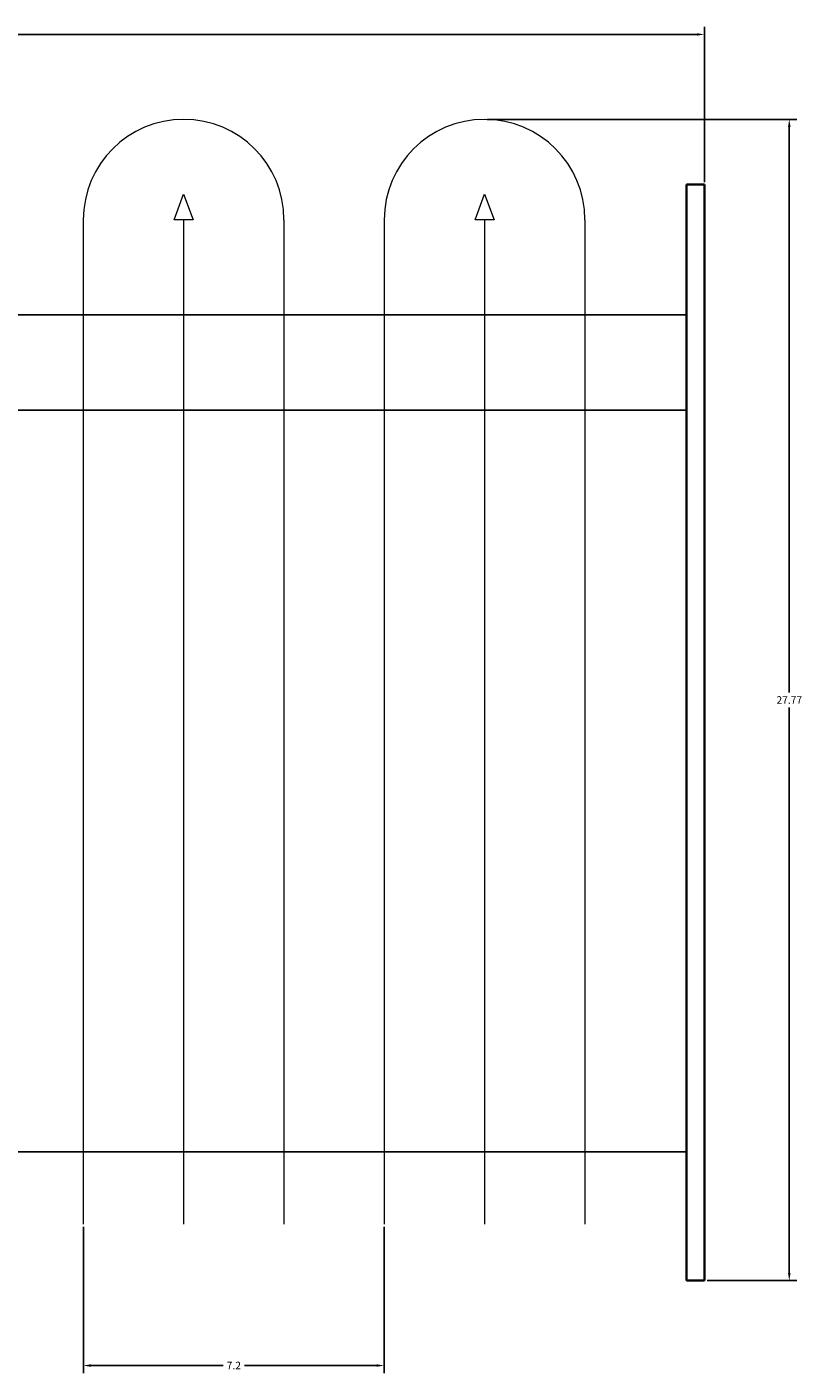
# Model space of a CAD drawing. Units: inches. Extents: x 756 to 915, y 488 to 695.
# Tile 12 of 25: x 794 to 813, y 592 to 624. Entities that reach past the tile are written whole.
import ezdxf

# ---------------------------------------------------------------- set-up
doc = ezdxf.new("R2010")
doc.units = ezdxf.units.IN
doc.header["$MEASUREMENT"] = 0
for name, color, linetype, lineweight in [('L-FENC-PCKT', 7, 'Continuous', 18), ('L-FENC-POST', 7, 'Continuous', 35), ('L-FENC-RAIL', 7, 'Continuous', 25), ('M-DIMS', 2, 'Continuous', 18)]:
    doc.layers.add(name, color=color, linetype=linetype, lineweight=lineweight)
doc.styles.get("Standard").update_dxf_attribs({"font": 'arial.ttf'})
doc.dimstyles.get("Standard").update_dxf_attribs({"dimtxt": 0.18, "dimasz": 0.18, "dimexe": 0.18, "dimexo": 0.0625, "dimgap": 0.09, "dimtad": 0, "dimtih": 1, "dimtoh": 1, "dimdec": 0, "dimzin": 0, "dimdsep": 46, "dimlunit": 3, "dimtxsty": 'Standard', "dimcen": 0.09, "dimadec": 0, "dimazin": 0, "dimtfac": 1, "dimtdec": 0, "dimtofl": 0, "dimtmove": 0, "dimatfit": 3, "dimfxl": 1, "dimtolj": 1, "dimtzin": 0, "dimarcsym": 0})

# ---------------------------------------------------------------- blocks, each defined once
blk = doc.blocks.new('FENCE-POST-RIGHT')
for p, q in [((0, 26.207), (0, 0)), ((0, 26.207), (0.427, 26.207)), ((0.427, 26.207), (0.427, 0)), ((0, 0), (0.427, 0))]:
    blk.add_line(p, q)
blk = doc.blocks.new('PICKET-ROUND-ARCH')
for p, q in [((0, 24.019), (0, 0)), ((4.8, 24.019), (4.8, 0))]:
    blk.add_line(p, q)
blk.add_arc((2.4, 24.019), 2.4, 0, 180)
blk = doc.blocks.new('PICKET-SPEAR-ARCH-INFILL')
blk.add_line((0.227, 24.019), (0.227, 0))
blk.add_lwpolyline([(0.227, 24.019), (0, 24.019), (0.227, 24.631), (0.455, 24.019)], close=True)
blk = doc.blocks.new('*D49')
at = {"layer": 'Defpoints', "color": 0, "transparency": 16777216}
for p in [(810.23, 623.683), (770.771, 620.092), (810.23, 620.092)]:
    blk.add_point(p, dxfattribs=at)
at = {"layer": 'M-DIMS', "color": 0, "lineweight": -2, "transparency": 16777216}
for p, q in [((770.771, 620.154), (770.771, 623.863)), ((810.23, 620.154), (810.23, 623.863)), ((770.951, 623.683), (790.107, 623.683)), ((810.05, 623.683), (790.894, 623.683))]:
    blk.add_line(p, q, dxfattribs=at)
at = {"layer": 'M-DIMS', "color": 0, "transparency": 16777216}
for points in [[(770.951, 623.713), (770.951, 623.653), (770.771, 623.683)], [(810.05, 623.713), (810.05, 623.653), (810.23, 623.683)]]:
    blk.add_solid(points, dxfattribs=at)
at = {"layer": 'M-DIMS', "color": 0, "transparency": 16777216, "insert": (790.5, 623.683), "char_height": 0.18, "attachment_point": 5}
blk.add_mtext('\\A1;39.46', dxfattribs=at)
blk = doc.blocks.new('*D50')
at = {"layer": 'Defpoints', "color": 0, "transparency": 16777216}
for p in [(804.969, 621.653), (812.26, 621.653), (810.23, 593.885)]:
    blk.add_point(p, dxfattribs=at)
at = {"layer": 'M-DIMS', "color": 0, "lineweight": -2, "transparency": 16777216}
for p, q in [((805.032, 621.653), (812.44, 621.653)), ((812.26, 621.473), (812.26, 607.949)), ((812.26, 594.065), (812.26, 607.588)), ((810.292, 593.885), (812.44, 593.885))]:
    blk.add_line(p, q, dxfattribs=at)
at = {"layer": 'M-DIMS', "color": 0, "transparency": 16777216}
for points in [[(812.23, 621.473), (812.29, 621.473), (812.26, 621.653)], [(812.23, 594.065), (812.29, 594.065), (812.26, 593.885)]]:
    blk.add_solid(points, dxfattribs=at)
at = {"layer": 'M-DIMS', "color": 0, "transparency": 16777216, "insert": (812.26, 607.769), "char_height": 0.18, "attachment_point": 5}
blk.add_mtext('\\A1;27.77', dxfattribs=at)
blk = doc.blocks.new('*D52')
at = {"layer": 'Defpoints', "color": 0, "transparency": 16777216}
for p in [(795.37, 595.234), (802.569, 595.234), (802.569, 591.855)]:
    blk.add_point(p, dxfattribs=at)
at = {"layer": 'M-DIMS', "color": 0, "lineweight": -2, "transparency": 16777216}
for p, q in [((795.37, 595.172), (795.37, 591.675)), ((802.569, 595.172), (802.569, 591.675)), ((795.55, 591.855), (798.717, 591.855)), ((802.389, 591.855), (799.222, 591.855))]:
    blk.add_line(p, q, dxfattribs=at)
at = {"layer": 'M-DIMS', "color": 0, "transparency": 16777216}
for points in [[(795.55, 591.885), (795.55, 591.825), (795.37, 591.855)], [(802.389, 591.885), (802.389, 591.825), (802.569, 591.855)]]:
    blk.add_solid(points, dxfattribs=at)
at = {"layer": 'M-DIMS', "color": 0, "transparency": 16777216, "insert": (798.97, 591.855), "char_height": 0.18, "attachment_point": 5}
blk.add_mtext('\\A1;7.2', dxfattribs=at)

msp = doc.modelspace()

# ---------------------------------------------------------------- linework, layer by layer
at = {"layer": 'L-FENC-RAIL'}
for p, q in [((771.198, 616.9765), (809.8029, 616.9765)), ((771.198, 614.7001), (809.8029, 614.7001)), ((771.198, 596.9663), (809.8029, 596.9663))]:
    msp.add_line(p, q, dxfattribs=at)

# ---------------------------------------------------------------- block references
at = {"layer": 'L-FENC-PCKT'}
for name, p in [('PICKET-ROUND-ARCH', (795.3692, 595.234)), ('PICKET-ROUND-ARCH', (802.5689, 595.234)), ('PICKET-SPEAR-ARCH-INFILL', (797.5422, 595.234)), ('PICKET-SPEAR-ARCH-INFILL', (804.7419, 595.234))]:
    msp.add_blockref(name, p, dxfattribs=at)
at = {"layer": 'L-FENC-POST', "rotation": 180}
msp.add_blockref('FENCE-POST-RIGHT', (810.2296, 620.0916), dxfattribs=at)

# ---------------------------------------------------------------- dimensions: what is measured, and where the dimension line sits
at = {"layer": 'M-DIMS'}
for base, p1, p2, override, picture, middle in [((810.2295, 623.6829), (770.7714, 620.0915), (810.2295, 620.0915), {"dimdec": 2, "dimlfac": 1, "dimrnd": 0, "dimzin": 0, "dimdsep": 46, "dimlunit": 2}, '*D49', (790.5004, 623.6829)), ((802.5694, 591.8547), (795.3697, 595.2343), (802.5694, 595.2343), {"dimdec": 1, "dimlfac": 1, "dimrnd": 0, "dimzin": 0, "dimdsep": 46, "dimlunit": 2}, '*D52', (798.9696, 591.8547))]:
    dim = msp.add_linear_dim(base=base, p1=p1, p2=p2, dimstyle='Standard', override=override, dxfattribs=at)
    dim.commit()
    dim.dimension.update_dxf_attribs({"geometry": picture, "text_midpoint": middle})
dim = msp.add_linear_dim(base=(812.2595, 621.6529), p1=(810.2295, 593.8847), p2=(804.9693, 621.6529), angle=90, dimstyle='Standard', override={"dimdec": 2, "dimlfac": 1, "dimrnd": 0, "dimzin": 0, "dimdsep": 46, "dimlunit": 2}, dxfattribs=at)
dim.commit()
dim.dimension.update_dxf_attribs({"geometry": '*D50', "text_midpoint": (812.2595, 607.7688)})

doc.saveas('drawing.dxf')
